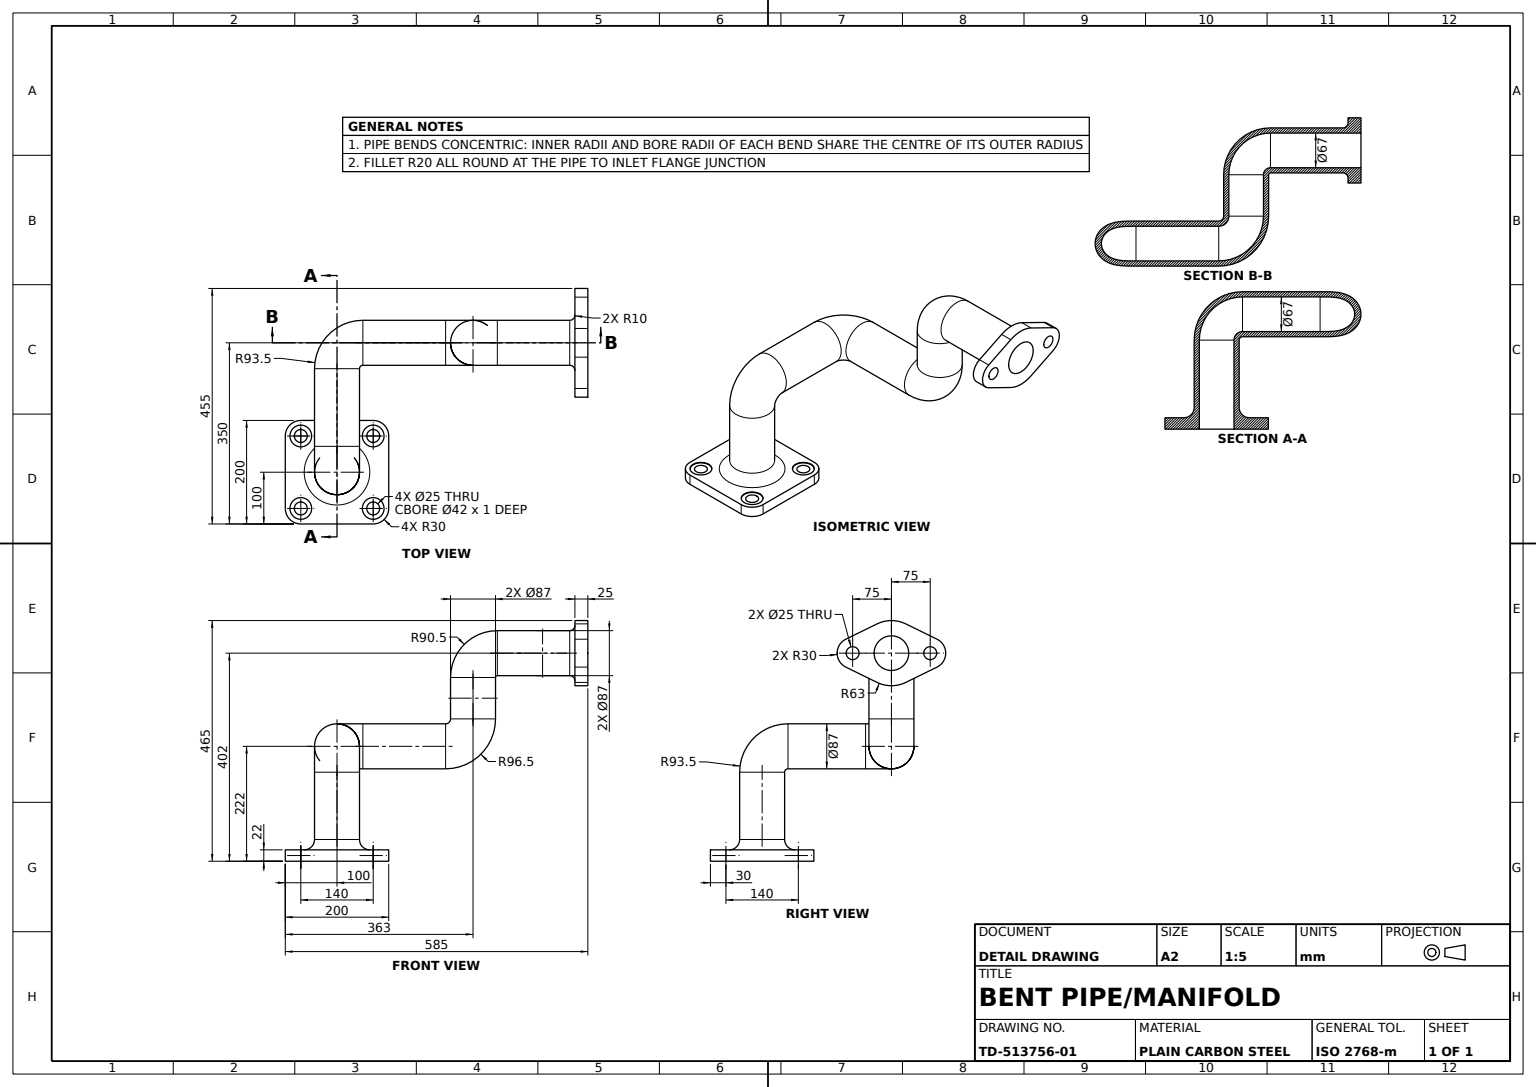
from build123d import *

# Parameters (mm, degrees)
INLET_FLANGE_SKETCH_R         = 12.5
INLET_FLANGE_200X200X22_DEPTH = 22
BOLT_SPOTFACE_SKETCH_R        = 21
BOLT_SPOTFACES_4X_42_DEPTH    = 1
INLET_BORE_SKETCH_R           = 33.5
INLET_BORE_67_DEPTH           = 25
PIPE_SECTION_1_PROFILE_R      = 43.5
PIPE_SECTION_1_PROFILE_R_2    = 33.5
PIPE_SECTION_2_PROFILE_R      = 43.5
PIPE_SECTION_2_PROFILE_R_2    = 33.5
S_BEND_PROFILE_R              = 43.5
S_BEND_PROFILE_R_2            = 33.5
OUTLET_START                  = 25
OUTLET_FLANGE_SKETCH_R        = 33.5
OUTLET_FLANGE_SKETCH_R_2      = 12.5
OUTLET_FLANGE_DEPTH           = 25
INLET_FLANGE_FILLET_R20_R     = 20
OUTLET_FILLET_R10_R           = 10


with BuildPart() as part:
    # Inlet Flange Sketch → Inlet Flange 200x200x22 (new body)
    with BuildSketch(Plane(origin=(0, 0, 0), x_dir=(1, 0, 0), z_dir=(0, 1, 0))):
        with BuildLine():
            Line((-70, 100), (70, 100))
            ThreePointArc((70, 100), (91.213203436, 91.213203436), (100, 70))
            Line((100, 70), (100, -70))
            ThreePointArc((100, -70), (91.213203436, -91.213203436), (70, -100))
            Line((70, -100), (-70, -100))
            ThreePointArc((-70, -100), (-91.213203436, -91.213203436), (-100, -70))
            Line((-100, -70), (-100, 70))
            ThreePointArc((-100, 70), (-91.213203436, 91.213203436), (-70, 100))
        make_face()
        with Locations(Location((-70, 70, 0), (0, 0, 270))):
            Circle(INLET_FLANGE_SKETCH_R, mode=Mode.SUBTRACT)
        with Locations(Location((70, 70, 0), (0, 0, 270))):
            Circle(INLET_FLANGE_SKETCH_R, mode=Mode.SUBTRACT)
        with Locations(Location((70, -70, 0), (0, 0, 270))):
            Circle(INLET_FLANGE_SKETCH_R, mode=Mode.SUBTRACT)
        with Locations(Location((-70, -70, 0), (0, 0, 270))):
            Circle(INLET_FLANGE_SKETCH_R, mode=Mode.SUBTRACT)
    extrude(amount=INLET_FLANGE_200X200X22_DEPTH)

    # Bolt Spotface Sketch → Bolt Spotfaces 4xØ42 (cut)
    with BuildSketch(Plane(origin=(0, 22, 0), x_dir=(1, 0, 0), z_dir=(0, 1, 0))):
        with Locations(Location((-70, 70, 0), (0, 0, 270))):
            Circle(BOLT_SPOTFACE_SKETCH_R)
        with Locations(Location((70, 70, 0), (0, 0, 270))):
            Circle(BOLT_SPOTFACE_SKETCH_R)
        with Locations(Location((70, -70, 0), (0, 0, 270))):
            Circle(BOLT_SPOTFACE_SKETCH_R)
        with Locations(Location((-70, -70, 0), (0, 0, 270))):
            Circle(BOLT_SPOTFACE_SKETCH_R)
    extrude(amount=-BOLT_SPOTFACES_4X_42_DEPTH, mode=Mode.SUBTRACT)

    # Inlet Bore Sketch → Inlet Bore Ø67 (cut)
    with BuildSketch(Plane(origin=(0, 22, 0), x_dir=(1, 0, 0), z_dir=(0, 1, 0))):
        with Locations(Location((0, 0, 0), (0, 0, 270))):
            Circle(INLET_BORE_SKETCH_R)
    extrude(amount=-INLET_BORE_67_DEPTH, mode=Mode.SUBTRACT)

    # Pipe Section 1: sweep along a path in Pipe Section 1 Path
    with BuildLine(Plane(origin=(0, 0, 0), x_dir=(0, 0, -1), z_dir=(1, 0, 0))) as pipe_section_1_path:
        Line((0, 22), (0, 172))
        ThreePointArc((0, 172), (14.644660941, 207.355339059), (50, 222))
        Line((50, 222), (180, 222))
    # Pipe Section 1 Profile → Pipe Section 1 (sweep)
    with BuildSketch(Plane(origin=(0, 22, 0), x_dir=(1, 0, 0), z_dir=(0, 1, 0))):
        Circle(PIPE_SECTION_1_PROFILE_R)
        Circle(PIPE_SECTION_1_PROFILE_R_2, mode=Mode.SUBTRACT)
    sweep(path=pipe_section_1_path.line)

    # Pipe Section 2: sweep along a path in Pipe Section 2 Path
    with BuildLine(Plane(origin=(0, 225, 0), x_dir=(1, 0, 0), z_dir=(0, 1, 0))) as pipe_section_2_path:
        Line((0, 180), (0, 200))
        ThreePointArc((0, 200), (14.644660941, 235.355339059), (50, 250))
        Line((50, 250), (200, 250))
    # Pipe Section 2 Profile → Pipe Section 2 (sweep)
    with BuildSketch(Plane(origin=(0, 0, -180), x_dir=(-1, 0, 0), z_dir=(0, 0, -1))):
        with Locations((0, 222)):
            Circle(PIPE_SECTION_2_PROFILE_R)
        with Locations((0, 222)):
            Circle(PIPE_SECTION_2_PROFILE_R_2, mode=Mode.SUBTRACT)
    sweep(path=pipe_section_2_path.line)

    # S-Bend Pipe Section: sweep along a path in S-Bend Path
    with BuildLine(Plane.XY.offset(-250)) as s_bend_pipe_section_path:
        Line((200, 225), (210, 225))
        ThreePointArc((210, 225), (245.355339059, 239.644660941), (260, 275))
        Line((260, 275), (260, 355))
        ThreePointArc((260, 355), (274.644660941, 390.355339059), (310, 405))
        Line((310, 405), (460, 405))
    # S-Bend Profile → S-Bend Pipe Section (sweep)
    with BuildSketch(Plane(origin=(200, 0, 0), x_dir=(0, 0, -1), z_dir=(1, 0, 0))):
        with Locations((250, 222)):
            Circle(S_BEND_PROFILE_R)
        with Locations((250, 222)):
            Circle(S_BEND_PROFILE_R_2, mode=Mode.SUBTRACT)
    sweep(path=s_bend_pipe_section_path.line)

    # Outlet Flange Sketch → Outlet Flange (add)
    with BuildSketch(Plane(origin=(460, 0, 0), x_dir=(0, 0, -1), z_dir=(1, 0, 0)).offset(OUTLET_START)):
        with BuildLine():
            Line((222.28, 458.573859688), (161.8, 428.939933185))
            ThreePointArc((161.8, 428.939933185), (145, 402), (161.8, 375.060066815))
            Line((161.8, 375.060066815), (222.28, 345.426140312))
            ThreePointArc((222.28, 345.426140312), (250, 339), (277.72, 345.426140312))
            Line((277.72, 345.426140312), (338.2, 375.060066815))
            ThreePointArc((338.2, 375.060066815), (355, 402), (338.2, 428.939933185))
            Line((338.2, 428.939933185), (277.72, 458.573859688))
            ThreePointArc((277.72, 458.573859688), (250, 465), (222.28, 458.573859688))
        make_face()
        with Locations((250, 402)):
            Circle(OUTLET_FLANGE_SKETCH_R, mode=Mode.SUBTRACT)
        with Locations((325, 402)):
            Circle(OUTLET_FLANGE_SKETCH_R_2, mode=Mode.SUBTRACT)
        with Locations((175, 402)):
            Circle(OUTLET_FLANGE_SKETCH_R_2, mode=Mode.SUBTRACT)
    extrude(amount=-OUTLET_FLANGE_DEPTH)

    # Inlet Flange Fillet R20
    inlet_flange_fillet_r20_edges = [part.edges().sort_by_distance(p)[0] for p in [
        (-43.5, 22, 0),
    ]]
    fillet(inlet_flange_fillet_r20_edges, radius=INLET_FLANGE_FILLET_R20_R)

    # Outlet Fillet R10
    outlet_fillet_r10_edges = [part.edges().sort_by_distance(p)[0] for p in [
        (460, 402, -206.5),
    ]]
    fillet(outlet_fillet_r10_edges, radius=OUTLET_FILLET_R10_R)


solid = part.part
